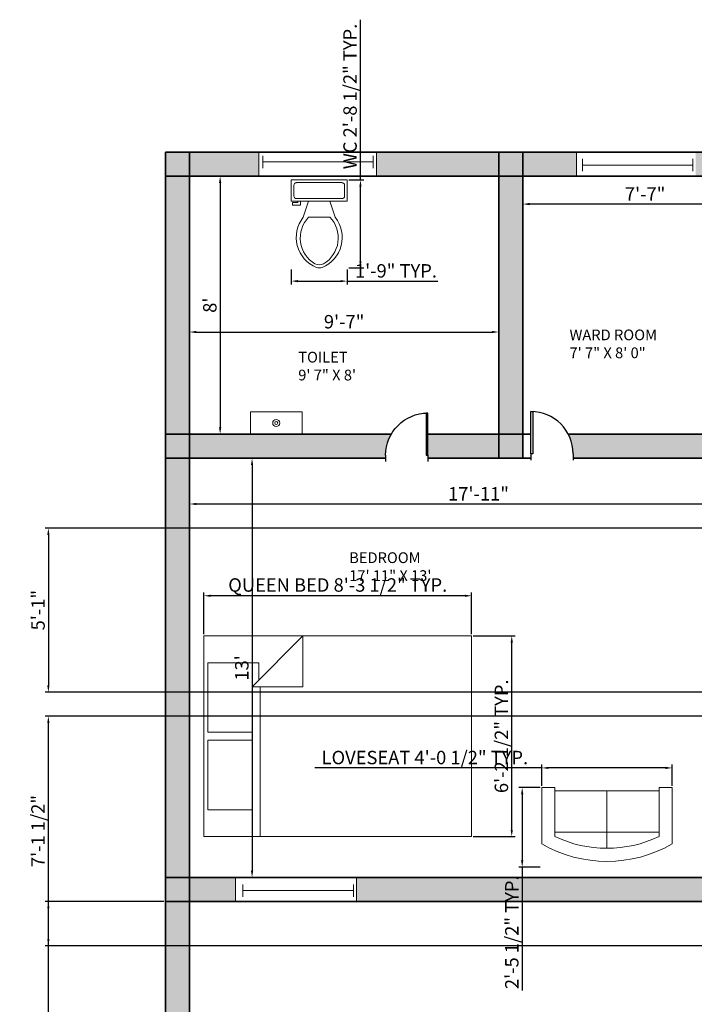
# Model space of a CAD drawing. Units: millimetres. Extents: x 2936 to 3516, y 349 to 1320.
# Tile 3 of 5: x 2936 to 3187, y 948 to 1315. Entities that reach past the tile are written whole.
import ezdxf

# ---------------------------------------------------------------- set-up
doc = ezdxf.new("R2010")
doc.units = ezdxf.units.MM
for name, color, linetype, lineweight in [('A-ANNO-DIMS', 3, 'Continuous', 13), ('A-AREA-IDEN', 190, 'Continuous', 18), ('A-FLOR-FIXT', 140, 'Continuous', 18), ('A-WALL-PATT', 50, 'Continuous', 13), ('doors', 10, 'Continuous', 25), ('furniture', 140, 'Continuous', 18), ('walls', 50, 'Continuous', 35), ('windows', 30, 'Continuous', 18)]:
    doc.layers.add(name, color=color, linetype=linetype, lineweight=lineweight)
doc.styles.get("Standard").update_dxf_attribs({"font": 'arial.ttf'})
doc.dimstyles.new('ISO-25', dxfattribs={"dimtxt": 5, "dimasz": 2.5, "dimexe": 1.25, "dimexo": 0.625, "dimtad": 1, "dimdec": 0, "dimlunit": 3, "dimtxsty": 'Standard', "dimcen": 2.5, "dimadec": 0, "dimazin": 0, "dimtfac": 1, "dimtdec": 0, "dimtmove": 0, "dimatfit": 3, "dimfxl": 1, "dimarcsym": 0})

# ---------------------------------------------------------------- blocks, each defined once
blk = doc.blocks.new('*U2')
for p, q in [((0, 0), (0, -6)), ((40, 0), (40, -6))]:
    blk.add_line(p, q)
blk.add_lwpolyline([(0, 0), (0, 40), (1.75, 40), (1.75, 0)], close=True)
blk.add_arc((0, 0), 40, 0, 90)
blk = doc.blocks.new('*U4')
for p, q in [((0, 4), (0, 0)), ((36, 4), (36, 0)), ((0, 2), (36, 2))]:
    blk.add_line(p, q)
blk = doc.blocks.new('Toilet - top')
for p, q in [((9.5, -6), (9.5, -2)), ((-10, -8.5), (-8, -8.5)), ((-10, -9.5), (-10, -8.5)), ((-7, -9.5), (-10, -9.5)), ((-8, -8.5), (-8, -8)), ((-7, -8), (-7, -9.5)), ((-4, -8), (-6, -14)), ((4, -8), (6, -14)), ((4, -14), (-4, -14))]:
    blk.add_line(p, q)
blk.add_lwpolyline([(10.5, -8), (10.5, 0), (-10.5, 0), (-10.5, -8)], close=True)
for points in [[(-9.5, -2), (-9.5, -6)], [(8.5, -1), (-8.5, -1)], [(-8.5, -7), (8.5, -7)]]:
    blk.add_lwpolyline(points)
for centre, radius, start, end in [((-8.62, -1.88), 0.884, 81.8699, 188.1301), ((8.62, -1.88), 0.884, 351.8699, 98.1301), ((-8.62, -6.12), 0.884, 171.8699, 278.1301), ((8.62, -6.12), 0.884, 261.8699, 8.1301), ((3.52, -21.58), 12.17, 141.4691, 247.9714), ((4.2, -21.82), 11.33, 136.3677, 238.9468), ((-3.52, -21.58), 12.17, 292.0284, 38.5307), ((-4.2, -21.82), 11.33, 301.053, 43.6321), ((0, -27.88), 4, 245.7318, 294.2682), ((0, -29), 4, 254.8605, 285.1395)]:
    blk.add_arc(centre, radius, start, end)
blk = doc.blocks.new('Bed - Queen')
for p, q in [((0, -80.00003), (0, 0)), ((0, 0), (59.99999, 0)), ((59.99999, 0), (59.99999, -80.00003)), ((7.99999, -1.2), (28.79998, -1.2)), ((7.99999, -14.4), (7.99999, -1.2)), ((28.79998, -1.2), (28.79998, -14.4)), ((31.19999, -1.2), (51.99999, -1.2)), ((31.19999, -14.4), (31.19999, -1.2)), ((51.99999, -1.2), (51.99999, -16.4)), ((0, -14.4), (44.8, -14.4)), ((59.99999, -29.6), (44.8, -14.4)), ((44.8, -14.4), (44.8, -29.6)), ((44.8, -16.8), (0, -16.8)), ((51.99999, -16.4), (46.79936, -16.4)), ((44.8, -29.6), (59.99999, -29.6)), ((59.99999, -80.00003), (0, -80.00003))]:
    blk.add_line(p, q)
blk = doc.blocks.new('Sofa - Roundback Loveseat 5 ft.')
for p, q in [((0, -32.44198), (0, -5.99998)), ((-24, -33.99998), (-24, -11.46958)), ((-23.9998, -13.38178), (23.99986, -13.38178)), ((24.00004, -33.99998), (24.00004, -11.46958)), ((-24, -32.44198), (24.00004, -32.44198))]:
    blk.add_line(p, q)
for points in [[(-24, -33.99998), (-30, -33.99998), (-30, -7.99998)], [(30.00004, -7.99998), (30.00004, -33.99998), (24.00004, -33.99998)]]:
    blk.add_lwpolyline(points)
for centre, radius, start, end in [((0, -60.24998), 60.24998, 60.13715, 119.8628), ((0, -61.38438), 55.38444, 64.32083, 115.6792)]:
    blk.add_arc(centre, radius, start, end)
blk = doc.blocks.new('*D15')
at = {"layer": 'A-ANNO-DIMS', "color": 0, "lineweight": -2, "transparency": 16777216}
for p, q in [((2999.19, 1198.91), (2999.19, 1199.54)), ((3114.19, 1198.91), (3114.19, 1199.54)), ((3001.69, 1198.29), (3111.69, 1198.29))]:
    blk.add_line(p, q, dxfattribs=at)
at = {"layer": 'A-ANNO-DIMS', "color": 0, "transparency": 16777216}
for points in [[(3001.69, 1198.71), (3001.69, 1197.87), (2999.19, 1198.29)], [(3111.69, 1198.71), (3111.69, 1197.87), (3114.19, 1198.29)]]:
    blk.add_solid(points, dxfattribs=at)
at = {"layer": 'Defpoints', "color": 0, "transparency": 16777216}
for p in [(2999.19, 1198.29), (3114.19, 1198.29), (3114.19, 1198.29)]:
    blk.add_point(p, dxfattribs=at)
at = {"layer": 'A-ANNO-DIMS', "color": 0, "transparency": 16777216, "insert": (3056.69, 1201.47), "char_height": 5, "attachment_point": 5}
blk.add_mtext('9\'-7"', dxfattribs=at)
blk = doc.blocks.new('*D16')
at = {"layer": 'A-ANNO-DIMS', "color": 0, "lineweight": -2, "transparency": 16777216}
for p, q in [((3006.6, 1256.28), (3011.8, 1256.28)), ((3010.55, 1253.78), (3010.55, 1162.78)), ((3006.6, 1160.28), (3011.8, 1160.28))]:
    blk.add_line(p, q, dxfattribs=at)
at = {"layer": 'A-ANNO-DIMS', "color": 0, "transparency": 16777216}
for points in [[(3010.13, 1253.78), (3010.97, 1253.78), (3010.55, 1256.28)], [(3010.13, 1162.78), (3010.97, 1162.78), (3010.55, 1160.28)]]:
    blk.add_solid(points, dxfattribs=at)
at = {"layer": 'Defpoints', "color": 0, "transparency": 16777216}
for p in [(3005.97, 1256.28), (3005.97, 1160.28), (3010.55, 1160.28)]:
    blk.add_point(p, dxfattribs=at)
at = {"layer": 'A-ANNO-DIMS', "color": 0, "transparency": 16777216, "insert": (3007.37, 1208.28), "char_height": 5, "attachment_point": 5, "rotation": 90}
blk.add_mtext("8'", dxfattribs=at)
blk = doc.blocks.new('*D18')
at = {"layer": 'A-ANNO-DIMS', "color": 0, "lineweight": -2, "transparency": 16777216}
for p, q in [((3123.19, 1246.53), (3123.19, 1247.16)), ((3214.19, 1246.53), (3214.19, 1247.16)), ((3211.69, 1245.91), (3125.69, 1245.91))]:
    blk.add_line(p, q, dxfattribs=at)
at = {"layer": 'A-ANNO-DIMS', "color": 0, "transparency": 16777216}
for points in [[(3125.69, 1246.32), (3125.69, 1245.49), (3123.19, 1245.91)], [(3211.69, 1246.32), (3211.69, 1245.49), (3214.19, 1245.91)]]:
    blk.add_solid(points, dxfattribs=at)
at = {"layer": 'Defpoints', "color": 0, "transparency": 16777216}
for p in [(3123.19, 1245.91), (3123.19, 1245.91), (3214.19, 1245.91)]:
    blk.add_point(p, dxfattribs=at)
at = {"layer": 'A-ANNO-DIMS', "color": 0, "transparency": 16777216, "insert": (3168.69, 1249.03), "char_height": 5, "attachment_point": 5}
blk.add_mtext('7\'-7"', dxfattribs=at)
blk = doc.blocks.new('*D23')
at = {"layer": 'A-ANNO-DIMS', "color": 0, "lineweight": -2, "transparency": 16777216}
for p, q in [((3030.54, 1151.28), (3021.18, 1151.28)), ((3022.43, 1148.78), (3022.43, 997.78)), ((3030.54, 995.28), (3021.18, 995.28))]:
    blk.add_line(p, q, dxfattribs=at)
at = {"layer": 'A-ANNO-DIMS', "color": 0, "transparency": 16777216}
for points in [[(3022.02, 1148.78), (3022.85, 1148.78), (3022.43, 1151.28)], [(3022.02, 997.78), (3022.85, 997.78), (3022.43, 995.28)]]:
    blk.add_solid(points, dxfattribs=at)
at = {"layer": 'Defpoints', "color": 0, "transparency": 16777216}
for p in [(3031.17, 1151.28), (3022.43, 995.28), (3031.17, 995.28)]:
    blk.add_point(p, dxfattribs=at)
at = {"layer": 'A-ANNO-DIMS', "color": 0, "transparency": 16777216, "insert": (3019.26, 1073.28), "char_height": 5, "attachment_point": 5, "rotation": 90}
blk.add_mtext("13'", dxfattribs=at)
blk = doc.blocks.new('*D24')
at = {"layer": 'A-ANNO-DIMS', "color": 0, "lineweight": -2, "transparency": 16777216}
for p, q in [((2999.19, 1134.91), (2999.19, 1135.53)), ((3211.69, 1134.28), (3001.69, 1134.28)), ((3214.19, 1134.91), (3214.19, 1135.53))]:
    blk.add_line(p, q, dxfattribs=at)
at = {"layer": 'A-ANNO-DIMS', "color": 0, "transparency": 16777216}
for points in [[(3001.69, 1134.7), (3001.69, 1133.87), (2999.19, 1134.28)], [(3211.69, 1134.7), (3211.69, 1133.87), (3214.19, 1134.28)]]:
    blk.add_solid(points, dxfattribs=at)
at = {"layer": 'Defpoints', "color": 0, "transparency": 16777216}
for p in [(2999.19, 1134.28), (2999.19, 1134.28), (3214.19, 1134.28)]:
    blk.add_point(p, dxfattribs=at)
at = {"layer": 'A-ANNO-DIMS', "color": 0, "transparency": 16777216, "insert": (3106.69, 1137.42), "char_height": 5, "attachment_point": 5}
blk.add_mtext('17\'-11"', dxfattribs=at)
blk = doc.blocks.new('*D39')
at = {"layer": 'A-ANNO-DIMS', "color": 0, "lineweight": -2, "transparency": 16777216}
for p, q in [((3004.51, 1085.81), (3004.51, 1101.38)), ((3101.62, 1100.13), (3007.01, 1100.13)), ((3104.12, 1085.81), (3104.12, 1101.38))]:
    blk.add_line(p, q, dxfattribs=at)
at = {"layer": 'A-ANNO-DIMS', "color": 0, "transparency": 16777216}
for points in [[(3007.01, 1100.54), (3007.01, 1099.71), (3004.51, 1100.13)], [(3101.62, 1100.54), (3101.62, 1099.71), (3104.12, 1100.13)]]:
    blk.add_solid(points, dxfattribs=at)
at = {"layer": 'Defpoints', "color": 0, "transparency": 16777216}
for p in [(3004.51, 1100.13), (3004.51, 1085.19), (3104.12, 1085.19)]:
    blk.add_point(p, dxfattribs=at)
at = {"layer": 'A-ANNO-DIMS', "color": 0, "transparency": 16777216, "insert": (3054.31, 1103.49), "char_height": 5, "attachment_point": 5}
blk.add_mtext('QUEEN BED 8\'-3 1/2" TYP.', dxfattribs=at)
blk = doc.blocks.new('*D40')
at = {"layer": 'A-ANNO-DIMS', "color": 0, "lineweight": -2, "transparency": 16777216}
for p, q in [((3104.74, 1085.19), (3120.31, 1085.19)), ((3119.06, 1012.98), (3119.06, 1082.69)), ((3104.74, 1010.48), (3120.31, 1010.48))]:
    blk.add_line(p, q, dxfattribs=at)
at = {"layer": 'A-ANNO-DIMS', "color": 0, "transparency": 16777216}
for points in [[(3118.64, 1082.69), (3119.47, 1082.69), (3119.06, 1085.19)], [(3118.64, 1012.98), (3119.47, 1012.98), (3119.06, 1010.48)]]:
    blk.add_solid(points, dxfattribs=at)
at = {"layer": 'Defpoints', "color": 0, "transparency": 16777216}
for p in [(3104.12, 1085.19), (3119.06, 1085.19), (3104.12, 1010.48)]:
    blk.add_point(p, dxfattribs=at)
at = {"layer": 'A-ANNO-DIMS', "color": 0, "transparency": 16777216, "insert": (3115.85, 1047.83), "char_height": 5, "attachment_point": 5, "rotation": 90}
blk.add_mtext('6\'-2 1/2" TYP.', dxfattribs=at)
blk = doc.blocks.new('*D41')
at = {"layer": 'A-ANNO-DIMS', "color": 0, "lineweight": -2, "transparency": 16777216}
for p, q in [((3130.22, 1029.4), (3130.22, 1037.31)), ((3178.75, 1029.4), (3178.75, 1037.31)), ((3130.22, 1036.06), (3045.74, 1036.06)), ((3176.25, 1036.06), (3132.72, 1036.06))]:
    blk.add_line(p, q, dxfattribs=at)
at = {"layer": 'A-ANNO-DIMS', "color": 0, "transparency": 16777216}
for points in [[(3132.72, 1036.47), (3132.72, 1035.64), (3130.22, 1036.06)], [(3176.25, 1036.47), (3176.25, 1035.64), (3178.75, 1036.06)]]:
    blk.add_solid(points, dxfattribs=at)
at = {"layer": 'Defpoints', "color": 0, "transparency": 16777216}
for p in [(3130.22, 1036.06), (3130.22, 1028.78), (3178.75, 1028.78)]:
    blk.add_point(p, dxfattribs=at)
at = {"layer": 'A-ANNO-DIMS', "color": 0, "transparency": 16777216, "insert": (3086.73, 1039.27), "char_height": 5, "attachment_point": 5}
blk.add_mtext('LOVESEAT 4\'-0 1/2" TYP.', dxfattribs=at)
blk = doc.blocks.new('*D42')
at = {"layer": 'A-ANNO-DIMS', "color": 0, "lineweight": -2, "transparency": 16777216}
for p, q in [((3129.59, 1028.78), (3121.69, 1028.78)), ((3122.94, 1026.28), (3122.94, 1001.62)), ((3129.59, 999.12), (3121.69, 999.12)), ((3122.94, 999.12), (3122.94, 953.16))]:
    blk.add_line(p, q, dxfattribs=at)
at = {"layer": 'A-ANNO-DIMS', "color": 0, "transparency": 16777216}
for points in [[(3122.52, 1026.28), (3123.36, 1026.28), (3122.94, 1028.78)], [(3122.52, 1001.62), (3123.36, 1001.62), (3122.94, 999.12)]]:
    blk.add_solid(points, dxfattribs=at)
at = {"layer": 'Defpoints', "color": 0, "transparency": 16777216}
for p in [(3130.22, 1028.78), (3122.94, 999.12), (3130.22, 999.12)]:
    blk.add_point(p, dxfattribs=at)
at = {"layer": 'A-ANNO-DIMS', "color": 0, "transparency": 16777216, "insert": (3119.73, 974.89), "char_height": 5, "attachment_point": 5, "rotation": 90}
blk.add_mtext('2\'-5 1/2" TYP.', dxfattribs=at)
blk = doc.blocks.new('*D43')
at = {"layer": 'A-ANNO-DIMS', "color": 0, "lineweight": -2, "transparency": 16777216}
for p, q in [((3062.75, 1254.87), (3062.75, 1314.53)), ((3058.47, 1254.87), (3064, 1254.87)), ((3062.75, 1224.64), (3062.75, 1252.37)), ((3058.47, 1222.14), (3064, 1222.14))]:
    blk.add_line(p, q, dxfattribs=at)
at = {"layer": 'A-ANNO-DIMS', "color": 0, "transparency": 16777216}
for points in [[(3062.34, 1252.37), (3063.17, 1252.37), (3062.75, 1254.87)], [(3062.34, 1224.64), (3063.17, 1224.64), (3062.75, 1222.14)]]:
    blk.add_solid(points, dxfattribs=at)
at = {"layer": 'Defpoints', "color": 0, "transparency": 16777216}
for p in [(3057.84, 1254.87), (3062.75, 1254.87), (3057.84, 1222.14)]:
    blk.add_point(p, dxfattribs=at)
at = {"layer": 'A-ANNO-DIMS', "color": 0, "transparency": 16777216, "insert": (3059.54, 1285.95), "char_height": 5, "attachment_point": 5, "rotation": 90}
blk.add_mtext('WC 2\'-8 1/2" TYP.', dxfattribs=at)
blk = doc.blocks.new('*D44')
at = {"layer": 'A-ANNO-DIMS', "color": 0, "lineweight": -2, "transparency": 16777216}
for p, q in [((3037.04, 1221.51), (3037.04, 1215.98)), ((3057.84, 1221.51), (3057.84, 1215.98)), ((3039.54, 1217.23), (3055.34, 1217.23)), ((3057.84, 1217.23), (3091.6, 1217.23))]:
    blk.add_line(p, q, dxfattribs=at)
at = {"layer": 'A-ANNO-DIMS', "color": 0, "transparency": 16777216}
for points in [[(3039.54, 1217.65), (3039.54, 1216.81), (3037.04, 1217.23)], [(3055.34, 1217.65), (3055.34, 1216.81), (3057.84, 1217.23)]]:
    blk.add_solid(points, dxfattribs=at)
at = {"layer": 'Defpoints', "color": 0, "transparency": 16777216}
for p in [(3037.04, 1222.14), (3057.84, 1222.14), (3057.84, 1217.23)]:
    blk.add_point(p, dxfattribs=at)
at = {"layer": 'A-ANNO-DIMS', "color": 0, "transparency": 16777216, "insert": (3075.97, 1220.41), "char_height": 5, "attachment_point": 5}
blk.add_mtext('1\'-9" TYP.', dxfattribs=at)
blk = doc.blocks.new('*D57')
at = {"layer": 'A-ANNO-DIMS', "color": 0, "lineweight": -2, "transparency": 16777216}
for p, q in [((2989.57, 986.28), (2945.39, 986.28)), ((2946.64, 819.36), (2946.64, 983.78)), ((2989.57, 816.86), (2945.39, 816.86))]:
    blk.add_line(p, q, dxfattribs=at)
at = {"layer": 'A-ANNO-DIMS', "color": 0, "transparency": 16777216}
for points in [[(2946.22, 983.78), (2947.06, 983.78), (2946.64, 986.28)], [(2946.22, 819.36), (2947.06, 819.36), (2946.64, 816.86)]]:
    blk.add_solid(points, dxfattribs=at)
at = {"layer": 'Defpoints', "color": 0, "transparency": 16777216}
for p in [(2946.64, 986.28), (2990.19, 986.28), (2990.19, 816.86)]:
    blk.add_point(p, dxfattribs=at)
at = {"layer": 'A-ANNO-DIMS', "color": 0, "transparency": 16777216, "insert": (2943.43, 901.57), "char_height": 5, "attachment_point": 5, "rotation": 90}
blk.add_mtext('14\'-1 1/2"', dxfattribs=at)
blk = doc.blocks.new('*D59')
at = {"layer": 'A-ANNO-DIMS', "color": 0, "lineweight": -2, "transparency": 16777216}
for p, q in [((3470.57, 1055.28), (2945.39, 1055.28)), ((2946.64, 972.36), (2946.64, 1052.78)), ((3470.57, 969.86), (2945.39, 969.86))]:
    blk.add_line(p, q, dxfattribs=at)
at = {"layer": 'A-ANNO-DIMS', "color": 0, "transparency": 16777216}
for points in [[(2946.22, 1052.78), (2947.06, 1052.78), (2946.64, 1055.28)], [(2946.22, 972.36), (2947.06, 972.36), (2946.64, 969.86)]]:
    blk.add_solid(points, dxfattribs=at)
at = {"layer": 'Defpoints', "color": 0, "transparency": 16777216}
for p in [(2946.64, 1055.28), (3471.19, 1055.28), (3471.19, 969.86)]:
    blk.add_point(p, dxfattribs=at)
at = {"layer": 'A-ANNO-DIMS', "color": 0, "transparency": 16777216, "insert": (2943.43, 1012.57), "char_height": 5, "attachment_point": 5, "rotation": 90}
blk.add_mtext('7\'-1 1/2"', dxfattribs=at)
blk = doc.blocks.new('*D65')
at = {"layer": 'A-ANNO-DIMS', "color": 0, "lineweight": -2, "transparency": 16777216}
for p, q in [((3213.57, 1125.28), (2945.39, 1125.28)), ((2946.64, 1122.78), (2946.64, 1066.78)), ((3213.57, 1064.28), (2945.39, 1064.28))]:
    blk.add_line(p, q, dxfattribs=at)
at = {"layer": 'A-ANNO-DIMS', "color": 0, "transparency": 16777216}
for points in [[(2946.22, 1122.78), (2947.06, 1122.78), (2946.64, 1125.28)], [(2946.22, 1066.78), (2947.06, 1066.78), (2946.64, 1064.28)]]:
    blk.add_solid(points, dxfattribs=at)
at = {"layer": 'Defpoints', "color": 0, "transparency": 16777216}
for p in [(3214.19, 1125.28), (2946.64, 1064.28), (3214.19, 1064.28)]:
    blk.add_point(p, dxfattribs=at)
at = {"layer": 'A-ANNO-DIMS', "color": 0, "transparency": 16777216, "insert": (2943.46, 1094.78), "char_height": 5, "attachment_point": 5, "rotation": 90}
blk.add_mtext('5\'-1"', dxfattribs=at)

msp = doc.modelspace()

# ---------------------------------------------------------------- hatches: boundary and pattern name
at = {"layer": 'A-WALL-PATT'}
h = msp.add_hatch(color=256, dxfattribs=at)
h.dxf.hatch_style = 1
h.paths.add_polyline_path([(2999.19, 1256.28), (2990.19, 1256.28), (2990.19, 1160.28), (2999.19, 1160.28)])
h.paths.add_polyline_path([(2999.19, 1265.28), (2990.19, 1265.28), (2990.19, 1256.28), (2999.19, 1256.28)])
h.paths.add_polyline_path([(3024.89, 1265.28), (2999.19, 1265.28), (2999.19, 1256.28), (3024.89, 1256.28)])
h.paths.add_polyline_path([(3074.24, 1160.28), (2999.19, 1160.28), (2999.19, 1151.28), (3072.14, 1151.28), (3072.14, 1152.43, -0.131652)])
h.paths.add_polyline_path([(2999.19, 1160.28), (2990.19, 1160.28), (2990.19, 1151.28), (2999.19, 1151.28)])
h.paths.add_polyline_path([(3123.19, 1256.28), (3114.19, 1256.28), (3114.19, 1160.28), (3123.19, 1160.28)])
h.paths.add_polyline_path([(3123.19, 1160.28), (3114.19, 1160.28), (3114.19, 1151.28), (3123.19, 1151.28)])
h.paths.add_polyline_path([(3114.19, 1160.28), (3087.85, 1160.28), (3087.85, 1152.43), (3087.85, 1151.28), (3114.19, 1151.28)])
h.paths.add_polyline_path([(3114.19, 1265.28), (3068.72, 1265.28), (3068.72, 1256.28), (3114.19, 1256.28)])
h.paths.add_polyline_path([(3123.19, 1265.28), (3114.19, 1265.28), (3114.19, 1256.28), (3123.19, 1256.28)])
h.paths.add_polyline_path([(3143.16, 1265.28), (3123.19, 1265.28), (3123.19, 1256.28), (3143.16, 1256.28)])
h.paths.add_polyline_path([(3214.19, 1265.28), (3187.49, 1265.28), (3187.49, 1256.28), (3214.19, 1256.28)])
h.paths.add_polyline_path([(3214.19, 1160.28), (3140.09, 1160.28, -0.121149), (3141.88, 1153), (3141.88, 1151.28), (3214.19, 1151.28)])
h.paths.add_polyline_path([(3223.19, 1256.28), (3214.19, 1256.28), (3214.19, 1160.28), (3223.19, 1160.28)])
h.paths.add_polyline_path([(3223.19, 1160.28), (3214.19, 1160.28), (3214.19, 1151.28), (3223.19, 1151.28)])
h.paths.add_polyline_path([(3223.19, 1151.28), (3214.19, 1151.28), (3214.19, 1134.28), (3223.19, 1134.28)])
h.paths.add_polyline_path([(3223.19, 1134.28), (3214.19, 1134.28), (3214.19, 1125.28), (3223.19, 1125.28)])
h.paths.add_polyline_path([(3223.19, 1125.28), (3214.19, 1125.28), (3214.19, 1064.28), (3223.19, 1064.28)])
h.paths.add_polyline_path([(3281.06, 1126.52, -0.130008), (3283.12, 1134.28), (3223.19, 1134.28), (3223.19, 1125.28), (3281.06, 1125.28)])
h.paths.add_polyline_path([(3223.19, 1265.28), (3214.19, 1265.28), (3214.19, 1256.28), (3223.19, 1256.28)])
h.paths.add_polyline_path([(3235.61, 1265.28), (3223.19, 1265.28), (3223.19, 1256.28), (3235.61, 1256.28)])
h.paths.add_polyline_path([(3297.19, 1265.28), (3278.85, 1265.28), (3278.85, 1256.28), (3297.19, 1256.28)])
h.paths.add_polyline_path([(3306.19, 1265.28), (3297.19, 1265.28), (3297.19, 1256.28), (3306.19, 1256.28)])
h.paths.add_polyline_path([(3306.19, 1256.28), (3297.19, 1256.28), (3297.19, 1134.28), (3306.19, 1134.28)])
h.paths.add_polyline_path([(3306.19, 1134.28), (3297.19, 1134.28), (3297.19, 1125.28), (3306.19, 1125.28)])
h.paths.add_polyline_path([(3306.19, 1125.28), (3297.19, 1125.28), (3297.19, 1084.87), (3305.61, 1084.87), (3306.19, 1084.87)])
h.paths.add_polyline_path([(3365.17, 1265.28), (3306.19, 1265.28), (3306.19, 1256.28), (3365.17, 1256.28)])
h.paths.add_polyline_path([(3462.19, 1265.28), (3409.24, 1265.28), (3409.24, 1256.28), (3462.19, 1256.28)])
h.paths.add_polyline_path([(3471.19, 1265.28), (3462.19, 1265.28), (3462.19, 1256.28), (3471.19, 1256.28)])
h.paths.add_polyline_path([(3471.19, 1256.28), (3462.19, 1256.28), (3462.19, 1225.41), (3471.19, 1225.41)])
h.paths.add_polyline_path([(3471.19, 1177.19), (3462.19, 1177.19), (3462.19, 1064.28), (3471.19, 1064.28)])
h.paths.add_polyline_path([(3462.19, 1064.28), (3368.33, 1064.28), (3368.33, 1055.28), (3462.19, 1055.28)])
h.paths.add_polyline_path([(3471.19, 1064.28), (3462.19, 1064.28), (3462.19, 1055.28), (3471.19, 1055.28)])
h.paths.add_polyline_path([(3471.19, 1055.28), (3462.19, 1055.28), (3462.19, 969.86), (3471.19, 969.86)])
h.paths.add_polyline_path([(3368.33, 1055.28), (3359.33, 1055.28), (3359.33, 995.28), (3368.33, 995.28)])
h.paths.add_polyline_path([(3368.33, 1064.28), (3359.33, 1064.28), (3359.33, 1055.28), (3368.33, 1055.28)])
h.paths.add_polyline_path([(3359.33, 995.28), (3306.19, 995.28), (3306.19, 986.28), (3359.33, 986.28)])
h.paths.add_polyline_path([(3368.33, 995.28), (3359.33, 995.28), (3359.33, 986.28), (3368.33, 986.28)])
h.paths.add_polyline_path([(3306.19, 995.28), (3297.19, 995.28), (3297.19, 986.28), (3306.19, 986.28)])
h.paths.add_polyline_path([(3306.19, 1011.04), (3298.85, 1011.04), (3297.19, 1011.04), (3297.19, 995.28), (3306.19, 995.28)])
h.paths.add_polyline_path([(3306.19, 1055.28), (3297.19, 1055.28), (3297.19, 1026.75), (3298.85, 1026.75, -0.122211), (3306.19, 1024.93)])
h.paths.add_polyline_path([(3306.19, 1064.28), (3297.19, 1064.28), (3297.19, 1055.28), (3306.19, 1055.28)])
h.paths.add_polyline_path([(3297.19, 1064.28), (3223.19, 1064.28), (3223.19, 1055.28), (3297.19, 1055.28)])
h.paths.add_polyline_path([(3223.19, 1064.28), (3214.19, 1064.28), (3214.19, 1055.28), (3223.19, 1055.28)])
h.paths.add_polyline_path([(3223.19, 1055.28), (3214.19, 1055.28), (3214.19, 1031.96), (3221.18, 1031.96), (3223.19, 1031.96)])
h.paths.add_polyline_path([(3223.19, 1016.25), (3221.18, 1016.25, -0.11578), (3214.19, 1017.89), (3214.19, 995.28), (3223.19, 995.28)])
h.paths.add_polyline_path([(3223.19, 995.28), (3214.19, 995.28), (3214.19, 986.28), (3223.19, 986.28)])
h.paths.add_polyline_path([(3214.19, 995.28), (3061.3, 995.28), (3061.3, 986.28), (3214.19, 986.28)])
h.paths.add_polyline_path([(2999.19, 1151.28), (2990.19, 1151.28), (2990.19, 995.28), (2999.19, 995.28)])
h.paths.add_polyline_path([(2999.19, 986.28), (2990.19, 986.28), (2990.19, 816.86), (2999.19, 816.86)])
h.paths.add_polyline_path([(2999.19, 995.28), (2990.19, 995.28), (2990.19, 986.28), (2999.19, 986.28)])
h.paths.add_polyline_path([(3016.23, 995.28), (2999.19, 995.28), (2999.19, 986.28), (3016.23, 986.28)])
h.paths.add_polyline_path([(2999.19, 807.86), (2990.19, 807.86), (2990.19, 683.86), (2999.19, 683.86)])
h.paths.add_polyline_path([(2999.19, 816.86), (2990.19, 816.86), (2990.19, 807.86), (2999.19, 807.86)])
h.paths.add_polyline_path([(3179.19, 816.86), (2999.19, 816.86), (2999.19, 807.86), (3179.19, 807.86)])
h.paths.add_polyline_path([(3188.19, 780.83), (3187.16, 780.83, -0.133677), (3179.19, 783), (3179.19, 683.86), (3188.19, 683.86)])
h.paths.add_polyline_path([(3188.19, 807.86), (3179.19, 807.86), (3179.19, 796.54), (3187.16, 796.54), (3188.19, 796.54)])
h.paths.add_polyline_path([(3188.19, 816.86), (3179.19, 816.86), (3179.19, 807.86), (3188.19, 807.86)])
h.paths.add_polyline_path([(3196.08, 816.86), (3188.19, 816.86), (3188.19, 807.86), (3196.08, 807.86)])
h.paths.add_polyline_path([(3321.19, 816.86), (3227.5, 816.86), (3227.5, 807.86), (3321.19, 807.86)])
h.paths.add_polyline_path([(3330.19, 867.56), (3321.19, 867.56), (3321.19, 816.86), (3330.19, 816.86)])
h.paths.add_polyline_path([(3330.19, 816.86), (3321.19, 816.86), (3321.19, 807.86), (3330.19, 807.86)])
h.paths.add_polyline_path([(3462.19, 816.86), (3330.19, 816.86), (3330.19, 807.86), (3462.19, 807.86)])
h.paths.add_polyline_path([(3471.19, 960.86), (3462.19, 960.86), (3462.19, 816.86), (3471.19, 816.86)])
h.paths.add_polyline_path([(3471.19, 816.86), (3462.19, 816.86), (3462.19, 807.86), (3471.19, 807.86)])
h.paths.add_polyline_path([(3471.19, 807.86), (3462.19, 807.86), (3462.19, 394.29), (3471.19, 394.29)])
h.paths.add_polyline_path([(3462.19, 715.94), (3227.5, 715.94), (3227.5, 708.13), (3227.5, 706.94), (3462.19, 706.94)])
h.paths.add_polyline_path([(3196.08, 715.94), (3188.19, 715.94), (3188.19, 706.94), (3196.08, 706.94), (3196.08, 708.13)])
h.paths.add_polyline_path([(2999.19, 674.86), (2990.19, 674.86), (2990.19, 554.86), (2999.19, 554.86)])
h.paths.add_polyline_path([(3179.19, 683.86), (2999.19, 683.86), (2999.19, 674.86), (3179.19, 674.86)])
h.paths.add_polyline_path([(2999.19, 683.86), (2990.19, 683.86), (2990.19, 674.86), (2999.19, 674.86)])
h.paths.add_polyline_path([(2999.19, 545.86), (2990.19, 545.86), (2990.19, 394.29), (2999.19, 394.29)])
h.paths.add_polyline_path([(3047.58, 554.86), (2999.19, 554.86), (2999.19, 545.86), (3047.58, 545.86)])
h.paths.add_polyline_path([(2999.19, 554.86), (2990.19, 554.86), (2990.19, 545.86), (2999.19, 545.86)])
h.paths.add_polyline_path([(3179.19, 554.86), (3096.19, 554.86), (3096.19, 545.86), (3179.19, 545.86)])
h.paths.add_polyline_path([(3188.19, 554.86), (3179.19, 554.86), (3179.19, 545.86), (3188.19, 545.86)])
h.paths.add_polyline_path([(3188.19, 652.99), (3187.11, 652.99, -0.132871), (3179.19, 655.13), (3179.19, 554.86), (3188.19, 554.86)])
h.paths.add_polyline_path([(3188.19, 683.86), (3179.19, 683.86), (3179.19, 674.86), (3188.19, 674.86)])
h.paths.add_polyline_path([(3188.19, 674.86), (3179.19, 674.86), (3179.19, 668.7), (3187.11, 668.7), (3188.19, 668.7)])
h.paths.add_polyline_path([(3462.19, 969.86), (3330.19, 969.86), (3330.19, 960.86), (3462.19, 960.86)])
h.paths.add_polyline_path([(3330.19, 969.86), (3321.19, 969.86), (3321.19, 960.86), (3330.19, 960.86)])
h.paths.add_polyline_path([(3330.19, 960.86), (3321.19, 960.86), (3321.19, 927.28), (3330.19, 927.28)])

# ---------------------------------------------------------------- linework, layer by layer
at = {"layer": 'A-FLOR-FIXT'}
msp.add_lwpolyline([(3021.81, 1160.28), (3041.05, 1160.28), (3041.05, 1168.57), (3021.81, 1168.57)], close=True, dxfattribs=at)
for radius in [1.33, 0.535]:
    msp.add_circle((3031.43, 1164.43), radius, dxfattribs=at)
at = {"layer": 'walls'}
for p, q in [((2990.19, 1265.28), (2990.19, 394.29)), ((2990.19, 1265.28), (3471.19, 1265.28)), ((2999.19, 1265.28), (2999.19, 394.29)), ((3114.19, 1265.28), (3114.19, 1151.28)), ((3123.19, 1265.28), (3123.19, 1151.28)), ((2990.19, 1256.28), (3471.19, 1256.28)), ((2990.19, 1160.28), (3074.24, 1160.28)), ((3087.85, 1160.28), (3126.17, 1160.28)), ((3140.09, 1160.28), (3223.19, 1160.28)), ((2990.19, 1151.28), (3072.14, 1151.28)), ((3087.85, 1151.28), (3126.17, 1151.28)), ((3141.88, 1151.28), (3223.19, 1151.28)), ((2990.19, 995.28), (3223.19, 995.28)), ((2990.19, 986.28), (3223.19, 986.28))]:
    msp.add_line(p, q, dxfattribs=at)
at = {"layer": 'windows'}
for p, q in [((3024.89, 1265.28), (3024.89, 1256.28)), ((3068.72, 1265.28), (3068.72, 1256.28)), ((3143.16, 1256.28), (3143.16, 1265.28)), ((3016.23, 995.28), (3016.23, 986.28)), ((3061.3, 995.28), (3061.3, 986.28))]:
    msp.add_line(p, q, dxfattribs=at)

# ---------------------------------------------------------------- block references
at = {"layer": 'A-FLOR-FIXT', "xscale": 0.9905491347394635, "yscale": 0.9905491347394635, "zscale": 0.9905491347394635}
msp.add_blockref('Toilet - top', (3047.44, 1254.87), dxfattribs=at)
at = {"layer": 'doors', "yscale": 0.3927729305520136, "zscale": 0.3927729305520136}
for p, xscale in [((3087.85, 1152.43), -0.3927729305520136), ((3126.17, 1153), 0.3927729305520136)]:
    msp.add_blockref('*U2', p, dxfattribs=dict(at, xscale=xscale))
at = {"layer": 'furniture'}
for name, p, xscale, yscale, zscale, rotation in [('Bed - Queen', (3004.51, 1010.48), 1.245124643961403, 1.245124643961403, 1.245124643961403, 90), ('Sofa - Roundback Loveseat 5 ft.', (3154.48, 1001.28), 0.8087673324917968, 0.8087673324917968, 0.8087673324917968, 180)]:
    msp.add_blockref(name, p, dxfattribs=dict(at, xscale=xscale, yscale=yscale, zscale=zscale, rotation=rotation))
at = {"layer": 'windows', "xscale": 1.142279500402185, "yscale": 1.142279500402185, "zscale": 1.142279500402185}
for p in [(3026.39, 1259.31), (3145.35, 1258.13), (3145.35, 1258.13), (3019.03, 988.11)]:
    msp.add_blockref('*U4', p, dxfattribs=at)

# ---------------------------------------------------------------- texts
at = {"layer": 'A-AREA-IDEN', "char_height": 4, "attachment_point": 1}
for s, width, insert in [('WARD ROOM \\P7\' 7" X 8\' 0"', 38.8147, (3140.55, 1199.22)), ('TOILET \\P9\' 7" X 8\'', 40.7391, (3039.62, 1190.94)), ('BEDROOM \\P17\' 11" X 13\' ', 48.902, (3058.59, 1116.3))]:
    msp.add_mtext_dynamic_manual_height_columns(s, width=width, gutter_width=12.5, heights=[0], dxfattribs=dict(at, insert=insert))

# ---------------------------------------------------------------- dimensions: what is measured, and where the dimension line sits
at = {"layer": 'A-ANNO-DIMS'}
for base, p1, p2, angle, text, picture, middle in [((3062.75, 1254.87), (3057.84, 1222.14), (3057.84, 1254.87), 90, 'WC <> TYP.', '*D43', (3059.54, 1285.95)), ((3004.51, 1100.13), (3104.12, 1085.19), (3004.51, 1085.19), 180, 'QUEEN BED <> TYP.', '*D39', (3054.31, 1103.49)), ((3119.06, 1085.19), (3104.12, 1010.48), (3104.12, 1085.19), 90, '<> TYP.', '*D40', (3115.85, 1047.83)), ((3130.22, 1036.06), (3178.75, 1028.78), (3130.22, 1028.78), 180, 'LOVESEAT <> TYP.', '*D41', (3086.73, 1039.27)), ((3122.94, 999.12), (3130.22, 1028.78), (3130.22, 999.12), 270, '<> TYP.', '*D42', (3119.73, 974.89))]:
    dim = msp.add_linear_dim(base=base, p1=p1, p2=p2, angle=angle, text=text, dimstyle='ISO-25', override={"dimdec": 1, "dimlfac": 1, "dimrnd": 0, "dimzin": 1, "dimdsep": 46, "dimlunit": 4, "dimfrac": 2}, dxfattribs=at)
    dim.commit()
    dim.dimension.update_dxf_attribs({"geometry": picture, "text_midpoint": middle})
for base, p1, p2, override, picture, middle in [((3010.55, 1160.28), (3005.97, 1256.28), (3005.97, 1160.28), {"dimclrd": 0, "dimclre": 0, "dimclrt": 0}, '*D16', (3007.37, 1208.28)), ((3022.43, 995.28), (3031.17, 1151.28), (3031.17, 995.28), {"dimclrd": 0, "dimclre": 0, "dimclrt": 0}, '*D23', (3019.26, 1073.28)), ((2946.64, 1064.28), (3214.19, 1125.28), (3214.19, 1064.28), {"dimdec": 1, "dimlfac": 1, "dimrnd": 0, "dimzin": 1, "dimdsep": 46, "dimlunit": 4, "dimfrac": 2}, '*D65', (2943.46, 1094.78)), ((2946.64, 1055.28), (3471.19, 969.86), (3471.19, 1055.28), {"dimdec": 1, "dimlfac": 1, "dimrnd": 0, "dimzin": 1, "dimdsep": 46, "dimlunit": 4, "dimfrac": 2}, '*D59', (2943.43, 1012.57)), ((2946.64, 986.28), (2990.19, 816.86), (2990.19, 986.28), {"dimdec": 1, "dimlfac": 1, "dimrnd": 0, "dimzin": 1, "dimdsep": 46, "dimlunit": 4, "dimfrac": 2}, '*D57', (2943.43, 901.57))]:
    dim = msp.add_linear_dim(base=base, p1=p1, p2=p2, angle=90, dimstyle='ISO-25', override=override, dxfattribs=at)
    dim.commit()
    dim.dimension.update_dxf_attribs({"geometry": picture, "text_midpoint": middle})
for base, p1, p2, picture, middle in [((3123.19, 1245.91), (3214.19, 1245.91), (3123.19, 1245.91), '*D18', (3168.69, 1249.03)), ((3114.19, 1198.29), (2999.19, 1198.29), (3114.19, 1198.29), '*D15', (3056.69, 1201.47)), ((2999.19, 1134.28), (3214.19, 1134.28), (2999.19, 1134.28), '*D24', (3106.69, 1137.42))]:
    dim = msp.add_linear_dim(base=base, p1=p1, p2=p2, dimstyle='ISO-25', override={"dimclrd": 0, "dimclre": 0, "dimclrt": 0}, dxfattribs=at)
    dim.commit()
    dim.dimension.update_dxf_attribs({"geometry": picture, "text_midpoint": middle})
dim = msp.add_linear_dim(base=(3057.84, 1217.23), p1=(3037.04, 1222.14), p2=(3057.84, 1222.14), text='<> TYP.', dimstyle='ISO-25', override={"dimdec": 1, "dimlfac": 1, "dimrnd": 0, "dimzin": 1, "dimdsep": 46, "dimlunit": 4, "dimfrac": 2}, dxfattribs=at)
dim.commit()
dim.dimension.update_dxf_attribs({"geometry": '*D44', "text_midpoint": (3075.97, 1220.41)})

doc.saveas('drawing.dxf')
